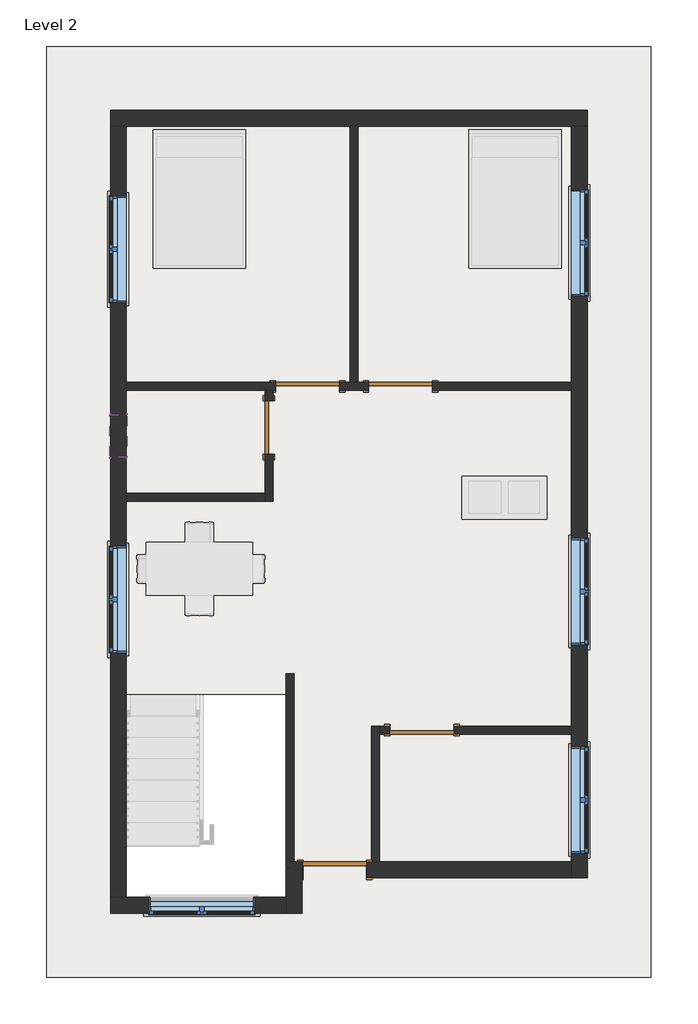
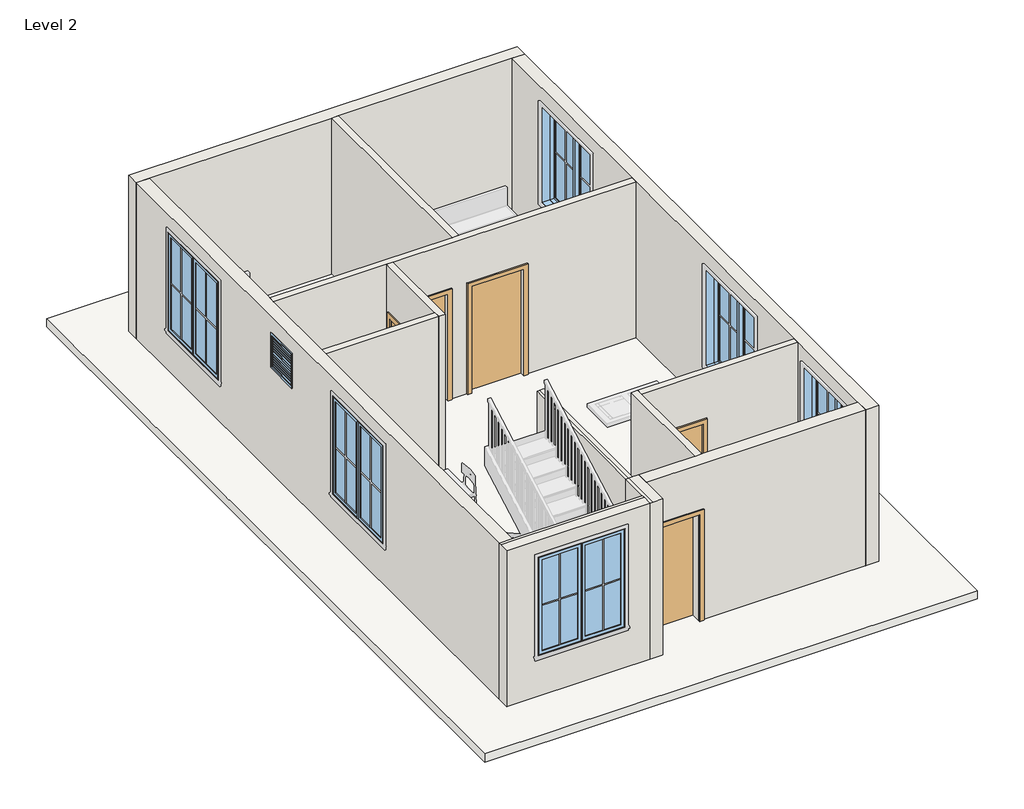
# One storey, part 1 of 3: 13 walls, 7 windows, 5 doors, 1 roof.
"""IFC4 building model written with IfcOpenShell, lengths in millimetres."""

from ifc_helpers import new_model, si_unit, frame, origin, place, context, project, spatial, polyline, outline, extrude, faceted_brep, transform, mapped, element, save
from components import door_214872d5, single_flush_door_3_e5f9f3c4, single_flush_door_3_305aa2a5, single_flush_door_3_0ca8825f, window_casement_double_win_5_f93960c7, window_f2d8fef0

model = new_model("IFC4")

# Units and contexts
model_context = context("Model", 3, world=origin())
ifc_project = project(units=[si_unit("LENGTHUNIT", "METRE", prefix="MILLI")], contexts=[model_context])

# Site, building, storey
site = spatial("IfcSite", under=ifc_project)
building = spatial("IfcBuilding", under=site)
storey = spatial("IfcBuildingStorey", under=building, Name="Level 2", Elevation=3048.0)

# Doors
placement = place(None, origin())
door_shape = door_214872d5(model_context)
element("IfcDoor", 1, ObjectType="Single-Flush : DOOR 2'6\"", at=placement, inside=storey, context=model_context, shape_type="MappedRepresentation", body=[
    mapped(door_shape, transform((-2193.930864, 251.0919982, 3048.0), x_axis=(0.0, 1.0, 0.0), y_axis=(-1.0, 0.0, 0.0), z_axis=(0.0, 0.0, 1.0))),
])
single_flush_door_3_shape = single_flush_door_3_e5f9f3c4(model_context)
element("IfcDoor", 2, ObjectType="Single-Flush : DOOR 3'", at=placement, inside=storey, context=model_context, shape_type="MappedRepresentation", body=[
    mapped(single_flush_door_3_shape, transform((-1641.3962678, 841.6419982, 3048.0), x_axis=(1.0, 0.0, 0.0), y_axis=(0.0, 1.0, 0.0), z_axis=(0.0, 0.0, 1.0))),
])
element("IfcDoor", 3, ObjectType="Single-Flush : DOOR 3'", at=placement, inside=storey, context=model_context, shape_type="MappedRepresentation", body=[
    mapped(single_flush_door_3_shape, transform((-3.180864, -4073.2580018, 3048.0), x_axis=(-1.0, 0.0, 0.0), y_axis=(0.0, -1.0, 0.0), z_axis=(0.0, 0.0, 1.0))),
])
single_flush_door_3_2_shape = single_flush_door_3_305aa2a5(model_context)
element("IfcDoor", 4, ObjectType="Single-Flush : DOOR 3'", at=placement, inside=storey, context=model_context, shape_type="MappedRepresentation", body=[
    mapped(single_flush_door_3_2_shape, transform((-307.980864, 841.6419982, 3048.0), x_axis=(-1.0, 0.0, 0.0), y_axis=(0.0, -1.0, 0.0), z_axis=(0.0, 0.0, 1.0))),
])
single_flush_door_3_3_shape = single_flush_door_3_0ca8825f(model_context)
element("IfcDoor", 5, ObjectType="Single-Flush : DOOR 3'", at=placement, inside=storey, context=model_context, shape_type="MappedRepresentation", body=[
    mapped(single_flush_door_3_3_shape, transform((-1250.955864, -6073.5080018, 3048.0), x_axis=(1.0, 0.0, 0.0), y_axis=(0.0, 1.0, 0.0), z_axis=(0.0, 0.0, 1.0))),
])

# Roof
element("IfcRoof", 6, ObjectType="ROOF 6\"", at=placement, inside=storey, context=model_context, shape_type="SweptSolid", body=[
    extrude(outline(polyline([(3273.419136, 5699.3919982), (3273.419136, -7610.2080018), (-5375.280864, -7610.2080018), (-5375.280864, 5699.3919982), (3273.419136, 5699.3919982)]), holes=[polyline([(-1895.480864, -3571.6080018), (-4232.280864, -3571.6080018), (-4232.280864, -6518.0080018), (-1895.480864, -6518.0080018), (-1895.480864, -3571.6080018)])]), frame((0.0, 0.0, 3048.0), z_axis=(0.0, 0.0, 1.0), x_axis=(1.0, 0.0, 0.0)), (0.0, 0.0, 1.0), 152.4),
])

# Walls
element("IfcWall", 7, ObjectType="WALL 4.5\"", at=placement, inside=storey, context=model_context, shape_type="SweptSolid", body=[
    extrude(outline(polyline([(-1031.880864, 898.7919982), (-1031.880864, 4556.3919982), (-917.580864, 4556.3919982), (-917.580864, 898.7919982), (-1031.880864, 898.7919982)])), frame((0.0, 0.0, 3048.0), z_axis=(0.0, 0.0, 1.0), x_axis=(1.0, 0.0, 0.0)), (0.0, 0.0, 1.0), 3048.0),
])
element("IfcWall", 8, ObjectType="WALL 4.5\"", at=placement, inside=storey, context=model_context, shape_type="Brep", body=[
    faceted_brep([(-765.180864, 898.7919982, 5181.6), (-765.180864, 898.7919982, 3048.0), (-917.580864, 898.7919982, 3048.0), (-1031.880864, 898.7919982, 3048.0), (-1184.1962678, 898.7919982, 3048.0), (-1184.1962678, 898.7919982, 5181.6), (-2098.5962678, 898.7919982, 5181.6), (-2098.5962678, 898.7919982, 3048.0), (-4232.280864, 898.7919982, 3048.0), (-4232.280864, 898.7919982, 6096.0), (-1031.880864, 898.7919982, 6096.0), (-917.580864, 898.7919982, 6096.0), (2130.419136, 898.7919982, 6096.0), (2130.419136, 898.7919982, 3048.0), (149.219136, 898.7919982, 3048.0), (149.219136, 898.7919982, 5181.6), (-1184.1962678, 784.4919982, 3048.0), (-765.180864, 784.4919982, 3048.0), (-765.180864, 784.4919982, 5181.6), (149.219136, 784.4919982, 5181.6), (149.219136, 784.4919982, 3048.0), (2130.419136, 784.4919982, 3048.0), (2130.419136, 784.4919982, 6096.0), (-2136.780864, 784.4919982, 6096.0), (-2251.080864, 784.4919982, 6096.0), (-4232.280864, 784.4919982, 6096.0), (-4232.280864, 784.4919982, 3048.0), (-2251.080864, 784.4919982, 3048.0), (-2136.780864, 784.4919982, 3048.0), (-2098.5962678, 784.4919982, 3048.0), (-2098.5962678, 784.4919982, 5181.6), (-1184.1962678, 784.4919982, 5181.6)], [[[0, 1, 2, 3, 4, 5, 6, 7, 8, 9, 10, 11, 12, 13, 14, 15]], [[16, 17, 18, 19, 20, 21, 22, 23, 24, 25, 26, 27, 28, 29, 30, 31]], [[29, 28, 27, 26, 8, 7]], [[14, 13, 21, 20]], [[4, 3, 2, 1, 17, 16]], [[13, 12, 22, 21]], [[9, 8, 26, 25]], [[5, 4, 16, 31]], [[6, 5, 31, 30]], [[7, 6, 30, 29]], [[18, 17, 1, 0]], [[19, 18, 0, 15]], [[20, 19, 15, 14]], [[12, 11, 10, 9, 25, 24, 23, 22]]]),
])
element("IfcWall", 9, ObjectType="WALL 4.5\"", at=placement, inside=storey, context=model_context, shape_type="Brep", body=[
    faceted_brep([(-2251.080864, 784.4919982, 3048.0), (-2251.080864, 632.0919982, 3048.0), (-2251.080864, 632.0919982, 5181.6), (-2251.080864, -129.9080018, 5181.6), (-2251.080864, -129.9080018, 3048.0), (-2251.080864, -688.7080018, 3048.0), (-2251.080864, -803.0080018, 3048.0), (-2251.080864, -803.0080018, 6096.0), (-2251.080864, -688.7080018, 6096.0), (-2251.080864, 784.4919982, 6096.0), (-2136.780864, 632.0919982, 5181.6), (-2136.780864, 632.0919982, 3048.0), (-2136.780864, 784.4919982, 3048.0), (-2136.780864, 784.4919982, 6096.0), (-2136.780864, -803.0080018, 6096.0), (-2136.780864, -803.0080018, 3048.0), (-2136.780864, -129.9080018, 3048.0), (-2136.780864, -129.9080018, 5181.6)], [[[0, 1, 2, 3, 4, 5, 6, 7, 8, 9]], [[10, 11, 12, 13, 14, 15, 16, 17]], [[16, 15, 6, 5, 4]], [[12, 11, 1, 0]], [[0, 9, 13, 12]], [[7, 6, 15, 14]], [[2, 1, 11, 10]], [[3, 2, 10, 17]], [[4, 3, 17, 16]], [[9, 8, 7, 14, 13]]]),
])
element("IfcWall", 10, ObjectType="WALL 4.5\"", at=placement, inside=storey, context=model_context, shape_type="SweptSolid", body=[
    extrude(outline(polyline([(-4232.280864, -688.7080018), (-2251.080864, -688.7080018), (-2251.080864, -803.0080018), (-4232.280864, -803.0080018), (-4232.280864, -688.7080018)])), frame((0.0, 0.0, 3048.0), z_axis=(0.0, 0.0, 1.0), x_axis=(1.0, 0.0, 0.0)), (0.0, 0.0, 1.0), 3048.0),
])
element("IfcWall", 11, ObjectType="WALL 4.5\"", at=placement, inside=storey, context=model_context, shape_type="Brep", body=[
    faceted_brep([(-1831.980864, -5959.2080018, 3048.0), (-1831.980864, -3266.8080018, 3048.0), (-1831.980864, -3266.8080018, 6096.0), (-1831.980864, -5959.2080018, 6096.0), (-1946.280864, -5959.2080018, 3048.0), (-1946.280864, -5959.2080018, 6096.0), (-1946.280864, -3266.8080018, 6096.0), (-1946.280864, -3266.8080018, 3048.0), (-1895.480864, -3266.8080018, 6096.0), (-1895.480864, -5959.2080018, 6096.0), (-1895.480864, -3571.6080018, 6096.0)], [[[0, 1, 2, 3]], [[4, 5, 6, 7]], [[1, 0, 4, 7]], [[2, 1, 7, 6, 8]], [[0, 3, 9, 5, 4]], [[3, 2, 8, 10, 9]], [[8, 6, 5, 9, 10]]]),
])
element("IfcWall", 12, ObjectType="WALL 4.5\"", at=placement, inside=storey, context=model_context, shape_type="Brep", body=[
    faceted_brep([(-612.780864, -5959.2080018, 3048.0), (-612.780864, -4130.4080018, 3048.0), (-612.780864, -4016.1080018, 3048.0), (-612.780864, -4016.1080018, 6096.0), (-612.780864, -4130.4080018, 6096.0), (-612.780864, -5959.2080018, 6096.0), (-727.080864, -5959.2080018, 3048.0), (-727.080864, -5959.2080018, 6096.0), (-727.080864, -4016.1080018, 6096.0), (-727.080864, -4016.1080018, 3048.0)], [[[0, 1, 2, 3, 4, 5]], [[6, 7, 8, 9]], [[2, 1, 0, 6, 9]], [[0, 5, 7, 6]], [[3, 2, 9, 8]], [[5, 4, 3, 8, 7]]]),
])
element("IfcWall", 13, ObjectType="WALL 4.5\"", at=placement, inside=storey, context=model_context, shape_type="SweptSolid", body=[
    extrude(outline(polyline([(3048.0, -612.780864), (3048.0, -460.380864), (5181.6, -460.380864), (5181.6, 454.019136), (3048.0, 454.019136), (3048.0, 2130.419136), (6096.0, 2130.419136), (6096.0, -612.780864), (3048.0, -612.780864)])), frame((0.0, -4130.4080018, 0.0), z_axis=(0.0, 1.0, 0.0), x_axis=(0.0, 0.0, 1.0)), (0.0, 0.0, 1.0), 114.3),
])
element("IfcWall", 14, ObjectType="WALL 9\"", at=placement, inside=storey, context=model_context, shape_type="Brep", body=[
    faceted_brep([(-4460.880864, 4556.3919982, 3048.0), (-4232.280864, 4556.3919982, 3048.0), (-1031.880864, 4556.3919982, 3048.0), (-917.580864, 4556.3919982, 3048.0), (2130.419136, 4556.3919982, 3048.0), (2359.019136, 4556.3919982, 3048.0), (2359.019136, 4556.3919982, 6096.0), (2130.419136, 4556.3919982, 6096.0), (-917.580864, 4556.3919982, 6096.0), (-1031.880864, 4556.3919982, 6096.0), (-4232.280864, 4556.3919982, 6096.0), (-4460.880864, 4556.3919982, 6096.0), (-4460.880864, 4784.9919982, 3048.0), (-4460.880864, 4784.9919982, 6096.0), (2359.019136, 4784.9919982, 6096.0), (2359.019136, 4784.9919982, 3048.0)], [[[0, 1, 2, 3, 4, 5, 6, 7, 8, 9, 10, 11]], [[12, 13, 14, 15]], [[5, 4, 3, 2, 1, 0, 12, 15]], [[6, 5, 15, 14]], [[0, 11, 13, 12]], [[11, 10, 9, 8, 7, 6, 14, 13]]]),
])
element("IfcWall", 15, ObjectType="WALL 9\"", at=placement, inside=storey, context=model_context, shape_type="Brep", body=[
    faceted_brep([(2130.419136, 4556.3919982, 3048.0), (2130.419136, 898.7919982, 3048.0), (2130.419136, 784.4919982, 3048.0), (2130.419136, -4016.1080018, 3048.0), (2130.419136, -4130.4080018, 3048.0), (2130.419136, -5959.2080018, 3048.0), (2130.419136, -6187.8080018, 3048.0), (2130.419136, -6187.8080018, 6096.0), (2130.419136, -5959.2080018, 6096.0), (2130.419136, -4130.4080018, 6096.0), (2130.419136, -4016.1080018, 6096.0), (2130.419136, 784.4919982, 6096.0), (2130.419136, 898.7919982, 6096.0), (2130.419136, 4556.3919982, 6096.0), (2130.419136, -5835.3830018, 5791.2), (2130.419136, -5835.3830018, 3962.4), (2130.419136, -4311.3830018, 3962.4), (2130.419136, -4311.3830018, 5791.2), (2130.419136, -2854.0580018, 5791.2), (2130.419136, -2854.0580018, 3962.4), (2130.419136, -1330.0580018, 3962.4), (2130.419136, -1330.0580018, 5791.2), (2130.419136, 2130.6919982, 5791.2), (2130.419136, 2130.6919982, 3962.4), (2130.419136, 3654.6919982, 3962.4), (2130.419136, 3654.6919982, 5791.2), (2359.019136, 4556.3919982, 3048.0), (2359.019136, 4556.3919982, 6096.0), (2359.019136, -6187.8080018, 6096.0), (2359.019136, -6187.8080018, 3048.0), (2359.019136, -5835.3830018, 5791.2), (2359.019136, -4311.3830018, 5791.2), (2359.019136, -4311.3830018, 3962.4), (2359.019136, -5835.3830018, 3962.4), (2359.019136, -2854.0580018, 5791.2), (2359.019136, -1330.0580018, 5791.2), (2359.019136, -1330.0580018, 3962.4), (2359.019136, -2854.0580018, 3962.4), (2359.019136, 2130.6919982, 5791.2), (2359.019136, 3654.6919982, 5791.2), (2359.019136, 3654.6919982, 3962.4), (2359.019136, 2130.6919982, 3962.4)], [[[0, 1, 2, 3, 4, 5, 6, 7, 8, 9, 10, 11, 12, 13], [14, 15, 16, 17], [18, 19, 20, 21], [22, 23, 24, 25]], [[26, 27, 28, 29], [30, 31, 32, 33], [34, 35, 36, 37], [38, 39, 40, 41]], [[6, 5, 4, 3, 2, 1, 0, 26, 29]], [[0, 13, 27, 26]], [[7, 6, 29, 28]], [[15, 14, 30, 33]], [[16, 15, 33, 32]], [[17, 16, 32, 31]], [[14, 17, 31, 30]], [[19, 18, 34, 37]], [[20, 19, 37, 36]], [[21, 20, 36, 35]], [[18, 21, 35, 34]], [[23, 22, 38, 41]], [[24, 23, 41, 40]], [[25, 24, 40, 39]], [[22, 25, 39, 38]], [[13, 12, 11, 10, 9, 8, 7, 28, 27]]]),
])
element("IfcWall", 16, ObjectType="WALL 9\"", at=placement, inside=storey, context=model_context, shape_type="Brep", body=[
    faceted_brep([(2130.419136, -5959.2080018, 3048.0), (-612.780864, -5959.2080018, 3048.0), (-727.080864, -5959.2080018, 3048.0), (-793.755864, -5959.2080018, 3048.0), (-793.755864, -5959.2080018, 5181.6), (-1708.155864, -5959.2080018, 5181.6), (-1708.155864, -5959.2080018, 3048.0), (-1717.680864, -5959.2080018, 3048.0), (-1717.680864, -5959.2080018, 6096.0), (-727.080864, -5959.2080018, 6096.0), (-612.780864, -5959.2080018, 6096.0), (2130.419136, -5959.2080018, 6096.0), (-793.755864, -6187.8080018, 5181.6), (-793.755864, -6187.8080018, 3048.0), (2130.419136, -6187.8080018, 3048.0), (2130.419136, -6187.8080018, 6096.0), (-1717.680864, -6187.8080018, 6096.0), (-1717.680864, -6187.8080018, 3048.0), (-1708.155864, -6187.8080018, 3048.0), (-1708.155864, -6187.8080018, 5181.6)], [[[0, 1, 2, 3, 4, 5, 6, 7, 8, 9, 10, 11]], [[12, 13, 14, 15, 16, 17, 18, 19]], [[18, 17, 7, 6]], [[14, 13, 3, 2, 1, 0]], [[0, 11, 15, 14]], [[8, 7, 17, 16]], [[4, 3, 13, 12]], [[5, 4, 12, 19]], [[6, 5, 19, 18]], [[11, 10, 9, 8, 16, 15]]]),
])
element("IfcWall", 17, ObjectType="WALL 9\"", at=placement, inside=storey, context=model_context, shape_type="Brep", body=[
    faceted_brep([(-1946.280864, -5959.2080018, 3048.0), (-1946.280864, -6467.2080018, 3048.0), (-1946.280864, -6695.8080018, 3048.0), (-1946.280864, -6695.8080018, 6096.0), (-1946.280864, -6467.2080018, 6096.0), (-1946.280864, -5959.2080018, 6096.0), (-1717.680864, -5959.2080018, 3048.0), (-1717.680864, -5959.2080018, 6096.0), (-1717.680864, -6187.8080018, 6096.0), (-1717.680864, -6695.8080018, 6096.0), (-1717.680864, -6695.8080018, 3048.0), (-1717.680864, -6187.8080018, 3048.0), (-1831.980864, -5959.2080018, 3048.0), (-1895.480864, -5959.2080018, 6096.0), (-1831.980864, -5959.2080018, 6096.0), (-1895.480864, -6695.8080018, 6096.0), (-1895.480864, -6518.0080018, 6096.0)], [[[0, 1, 2, 3, 4, 5]], [[6, 7, 8, 9, 10, 11]], [[2, 1, 0, 12, 6, 11, 10]], [[0, 5, 13, 14, 7, 6, 12]], [[3, 2, 10, 9, 15]], [[5, 4, 3, 15, 16, 13]], [[15, 9, 8, 7, 14, 13, 16]]]),
])
element("IfcWall", 18, ObjectType="WALL 9\"", at=placement, inside=storey, context=model_context, shape_type="Brep", body=[
    faceted_brep([(-1946.280864, -6467.2080018, 3048.0), (-4232.280864, -6467.2080018, 3048.0), (-4460.880864, -6467.2080018, 3048.0), (-4460.880864, -6467.2080018, 6096.0), (-4232.280864, -6467.2080018, 6096.0), (-1946.280864, -6467.2080018, 6096.0), (-3914.780864, -6467.2080018, 5791.2), (-3914.780864, -6467.2080018, 3962.4), (-2390.780864, -6467.2080018, 3962.4), (-2390.780864, -6467.2080018, 5791.2), (-1946.280864, -6695.8080018, 3048.0), (-1946.280864, -6695.8080018, 6096.0), (-4460.880864, -6695.8080018, 6096.0), (-4460.880864, -6695.8080018, 3048.0), (-3914.780864, -6695.8080018, 5791.2), (-2390.780864, -6695.8080018, 5791.2), (-2390.780864, -6695.8080018, 3962.4), (-3914.780864, -6695.8080018, 3962.4), (-1946.280864, -6518.0080018, 6096.0), (-4460.880864, -6518.0080018, 6096.0), (-4232.280864, -6518.0080018, 6096.0)], [[[0, 1, 2, 3, 4, 5], [6, 7, 8, 9]], [[10, 11, 12, 13], [14, 15, 16, 17]], [[2, 1, 0, 10, 13]], [[0, 5, 18, 11, 10]], [[3, 2, 13, 12, 19]], [[7, 6, 14, 17]], [[8, 7, 17, 16]], [[9, 8, 16, 15]], [[6, 9, 15, 14]], [[5, 4, 3, 19, 20, 18]], [[19, 12, 11, 18, 20]]]),
])
element("IfcWall", 19, ObjectType="WALL 9\"", at=placement, inside=storey, context=model_context, shape_type="Brep", body=[
    faceted_brep([(-4232.280864, -6467.2080018, 3048.0), (-4232.280864, -803.0080018, 3048.0), (-4232.280864, -688.7080018, 3048.0), (-4232.280864, 784.4919982, 3048.0), (-4232.280864, 898.7919982, 3048.0), (-4232.280864, 4556.3919982, 3048.0), (-4232.280864, 4556.3919982, 6096.0), (-4232.280864, 898.7919982, 6096.0), (-4232.280864, 784.4919982, 6096.0), (-4232.280864, -688.7080018, 6096.0), (-4232.280864, -803.0080018, 6096.0), (-4232.280864, -3571.6080018, 6096.0), (-4232.280864, -6467.2080018, 6096.0), (-4232.280864, -1445.1400081, 5791.2), (-4232.280864, -1445.1400081, 3962.4), (-4232.280864, -2969.1400081, 3962.4), (-4232.280864, -2969.1400081, 5791.2), (-4232.280864, 3562.6287133, 5791.2), (-4232.280864, 3562.6287133, 3962.4), (-4232.280864, 2038.6287133, 3962.4), (-4232.280864, 2038.6287133, 5791.2), (-4232.280864, -174.3580018, 5791.2), (-4232.280864, 435.2419982, 5791.2), (-4232.280864, 435.2419982, 5181.6), (-4232.280864, -174.3580018, 5181.6), (-4460.880864, -6467.2080018, 3048.0), (-4460.880864, -6467.2080018, 6096.0), (-4460.880864, 4556.3919982, 6096.0), (-4460.880864, 4556.3919982, 3048.0), (-4460.880864, -1445.1400081, 5791.2), (-4460.880864, -2969.1400081, 5791.2), (-4460.880864, -2969.1400081, 3962.4), (-4460.880864, -1445.1400081, 3962.4), (-4460.880864, 3562.6287133, 5791.2), (-4460.880864, 2038.6287133, 5791.2), (-4460.880864, 2038.6287133, 3962.4), (-4460.880864, 3562.6287133, 3962.4), (-4460.880864, -174.3580018, 5791.2), (-4460.880864, -174.3580018, 5181.6), (-4460.880864, 435.2419982, 5181.6), (-4460.880864, 435.2419982, 5791.2)], [[[0, 1, 2, 3, 4, 5, 6, 7, 8, 9, 10, 11, 12], [13, 14, 15, 16], [17, 18, 19, 20], [21, 22, 23, 24]], [[25, 26, 27, 28], [29, 30, 31, 32], [33, 34, 35, 36], [37, 38, 39, 40]], [[5, 4, 3, 2, 1, 0, 25, 28]], [[6, 5, 28, 27]], [[0, 12, 26, 25]], [[14, 13, 29, 32]], [[15, 14, 32, 31]], [[16, 15, 31, 30]], [[13, 16, 30, 29]], [[18, 17, 33, 36]], [[19, 18, 36, 35]], [[20, 19, 35, 34]], [[17, 20, 34, 33]], [[38, 37, 21, 24]], [[39, 38, 24, 23]], [[40, 39, 23, 22]], [[37, 40, 22, 21]], [[12, 11, 10, 9, 8, 7, 6, 27, 26]]]),
])

# Windows
window_casement_double_win_5_shape = window_casement_double_win_5_f93960c7(model_context)
element("IfcWindow", 20, ObjectType="Window-Casement-Double : WIN 5'", at=placement, inside=storey, context=model_context, shape_type="MappedRepresentation", body=[
    mapped(window_casement_double_win_5_shape, transform((-3152.780864, -6581.5080018, 3048.0), x_axis=(-1.0, 0.0, 0.0), y_axis=(0.0, -1.0, 0.0), z_axis=(0.0, 0.0, 1.0))),
])
element("IfcWindow", 21, ObjectType="Window-Casement-Double : WIN 5'", at=placement, inside=storey, context=model_context, shape_type="MappedRepresentation", body=[
    mapped(window_casement_double_win_5_shape, transform((2244.719136, -5073.3830018, 3048.0), x_axis=(0.0, -1.0, 0.0), y_axis=(1.0, 0.0, 0.0), z_axis=(0.0, 0.0, 1.0))),
])
element("IfcWindow", 22, ObjectType="Window-Casement-Double : WIN 5'", at=placement, inside=storey, context=model_context, shape_type="MappedRepresentation", body=[
    mapped(window_casement_double_win_5_shape, transform((2244.719136, -2092.0580018, 3048.0), x_axis=(0.0, -1.0, 0.0), y_axis=(1.0, 0.0, 0.0), z_axis=(0.0, 0.0, 1.0))),
])
element("IfcWindow", 23, ObjectType="Window-Casement-Double : WIN 5'", at=placement, inside=storey, context=model_context, shape_type="MappedRepresentation", body=[
    mapped(window_casement_double_win_5_shape, transform((-4346.580864, -2207.1400081, 3048.0), x_axis=(0.0, 1.0, 0.0), y_axis=(-1.0, 0.0, 0.0), z_axis=(0.0, 0.0, 1.0))),
])
element("IfcWindow", 24, ObjectType="Window-Casement-Double : WIN 5'", at=placement, inside=storey, context=model_context, shape_type="MappedRepresentation", body=[
    mapped(window_casement_double_win_5_shape, transform((2244.719136, 2892.6919982, 3048.0), x_axis=(0.0, -1.0, 0.0), y_axis=(1.0, 0.0, 0.0), z_axis=(0.0, 0.0, 1.0))),
])
element("IfcWindow", 25, ObjectType="Window-Casement-Double : WIN 5'", at=placement, inside=storey, context=model_context, shape_type="MappedRepresentation", body=[
    mapped(window_casement_double_win_5_shape, transform((-4346.580864, 2800.6287133, 3048.0), x_axis=(0.0, 1.0, 0.0), y_axis=(-1.0, 0.0, 0.0), z_axis=(0.0, 0.0, 1.0))),
])
window_shape = window_f2d8fef0(model_context)
element("IfcWindow", 26, ObjectType="Window-Louvers : 24\" x 24\"", at=placement, inside=storey, context=model_context, shape_type="MappedRepresentation", body=[
    mapped(window_shape, transform((-4352.930864, 130.4419982, 4267.2), x_axis=(0.0, 1.0, 0.0), y_axis=(-1.0, 0.0, 0.0), z_axis=(0.0, 0.0, 1.0))),
])

save(model, "model.ifc")

# Revit data of these elements
# Type "Single-Flush : DOOR 2'6\""
#   Type Mark = "9"
#   Construction Type Id = "MDOOR"
#   Assembly Code = "C1020"
#   Analytic Construction = "Metal"
#   Thickness = 0' - 2"
#   Heat Transfer Coefficient (U) = 0.651978 BTU/(h·ft²·°F)
#   Height = 7' - 0"
#   Trim Projection Ext = 0' - 1"
#   Trim Projection Int = 0' - 1"
#   Trim Width = 0' - 3"
#   Width = 2' - 6"
#   Define Thermal Properties by = 1
#   Door Material = Door - Panel
#   Frame Material = Door - Frame
#   Visual Light Transmittance = 0
#   Solar Heat Gain Coefficient = 0
#   Function = (empty or 0)
#   Wall Closure = (empty or 0)
# Type "Single-Flush : DOOR 3'"
#   Type Mark = "8"
#   Construction Type Id = "MDOOR"
#   Assembly Code = "C1020"
#   Analytic Construction = "Metal"
#   Thickness = 0' - 2"
#   Heat Transfer Coefficient (U) = 0.651978 BTU/(h·ft²·°F)
#   Height = 7' - 0"
#   Trim Projection Ext = 0' - 1"
#   Trim Projection Int = 0' - 1"
#   Trim Width = 0' - 3"
#   Width = 3' - 0"
#   Define Thermal Properties by = 1
#   Door Material = Door - Panel
#   Frame Material = Door - Frame
#   Visual Light Transmittance = 0
#   Solar Heat Gain Coefficient = 0
#   Function = (empty or 0)
#   Wall Closure = (empty or 0)
# Type "ROOF 6\""
#   Assembly Code = "B1020"
#   Layers, outside or top first: 0' - 6" no material (function 1)
# Type "WALL 4.5\""
#   Assembly Code = "B2010"
#   Layers, outside or top first: 0' - 4 1/2" no material (function 1)
# Type "WALL 9\""
#   Assembly Code = "B2010"
#   Layers, outside or top first: 0' - 9" no material (function 1)
# Type "Window-Casement-Double : WIN 5'"
#   Type Mark = "18"
#   Fire Rating = "0.5h"
#   Assembly Code = "B2020100"
#   Analytic Construction = "Double glazing - domestic"
#   Frame Extension [instance default] = 0' - 0 1/4"
#   Window Inset [instance default] = 0' - 0"
#   Wall Thickness [instance default] = 0' - 6"
#   Interior Wall Closure [instance default] = 0' - 2 1/4"
#   Half Width = 2' - 6"
#   Visual Light Transmittance = 0.81
#   Thermal Resistance (R) = 1.8146 (h·ft²·°F)/BTU
#   Solar Heat Gain Coefficient = 0.76
#   Rough Width = 5' - 0 1/2"
#   Rough Height = 6' - 0 1/2"
#   Height = 6' - 0"
#   Heat Transfer Coefficient (U) = 0.5511 BTU/(h·ft²·°F)
#   Exterior Wall Closure [instance default] = 0' - 1 1/4"
#   Extension Jamb [instance default] = 0' - 2 1/4"
#   Default Sill Height = 3' - 0"
#   Width = 5' - 0"
#   Muntin Visibility = yes
#   Interior Trim Visibility [instance default] = yes
#   Exterior Trim Visibility [instance default] = yes
#   Extension Jamb Visibility [instance default] = yes
#   Interior Trim Material = Wood - Stained
#   Muntin Pattern = Muntin Pattern_2x2 : Muntin Pattern_2x2
#   Interior Trim = Trim-Window-Interior-Flat : Picture Frame
#   Interior Frame Material = Wood - Stained
#   Glass Panel Material = Glass
#   Exterior Trim Material = Clad - White
#   Exterior Trim = Trim-Window-Exterior-Flat : with Sill
#   Exterior Frame Material = Clad - White
#   Wall Closure = (empty or 0)
# Type "Window-Louvers : 24\" x 24\""
#   Type Mark = "19"
#   Construction Type Id = "GSP4R"
#   Assembly Code = "B20"
#   Analytic Construction = "1/8 in Pilkington single glazing"
#   Visual Light Transmittance = 0.9
#   Thermal Resistance (R) = 1.53941 (h·ft²·°F)/BTU
#   Solar Heat Gain Coefficient = 0.78
#   Max Height = 1' - 11.74264"
#   Height = 2' - 0"
#   Heat Transfer Coefficient (U) = 0.6496 BTU/(h·ft²·°F)
#   Blade Width [instance default] = 1' - 10 1/2"
#   Blade Vertical Thickness = 0' - 0.35355"
#   Blade Thickness = 0' - 0 1/4"
#   Blade Spacing = 0' - 1 1/2"
#   Blade Height = 0' - 1.85355"
#   Blade Depth = 0' - 3"
#   Blade Angle = 45.00°
#   Default Sill Height = 3' - 0"
#   Trim Projection_Exterior = 0' - 0 1/2"
#   Trim Projection_Interior = 0' - 0 1/2"
#   Trim Width_Exterior = 0' - 1 1/2"
#   Trim Width_Interior = 0' - 1 1/2"
#   Width = 2' - 0"
#   Max Blade Count = 12
#   Define Thermal Properties by = 1
#   Blade Count = 12
#   Frame Material = Birch
#   Louver Material = Birch
#   Trim Exterior Material = Birch
#   Trim Interior Material = Birch
#   Wall Closure = (empty or 0)
# Element 1 (IfcDoor, "Single-Flush : DOOR 2'6\"")
#   Phase Created = New Construction
#   Materials on its faces: "Door - Frame", "Door - Panel"
# Elements 2, 3, 4, 5 (IfcDoor, "Single-Flush : DOOR 3'")
#   Phase Created = New Construction
#   Materials on its faces: "Door - Frame", "Door - Panel"
# Element 6 (IfcRoof, "ROOF 6\"")
#   built-in parameter 1001705 = 10.5 (stored number, unit not read)
#   built-in parameter 1001710 = 33615
#   Phase Created = New Construction
#   Materials on its faces: "Copper", "Wood - Stained"
# Elements 7, 8, 9, 10, 12, 13 (IfcWall, "WALL 4.5\"")
#   Top Offset = 0' - 0"
#   Base Offset = 0' - 0"
#   Unconnected Height = 10' - 0"
#   wall height = 10' - 0"
#   Phase Created = New Construction
#   Base Constraint = Level 2
#   Materials on its faces: "Default Wall"
# Element 11 (IfcWall, "WALL 4.5\"")
#   Top Offset = 0' - 0"
#   Base Offset = 0' - 0"
#   Unconnected Height = 10' - 0"
#   wall height = 10' - 0"
#   Phase Created = New Construction
#   Base Constraint = Level 2
#   Materials on its faces: "Default Wall", "Copper"
# Elements 14, 15, 16 (IfcWall, "WALL 9\"")
#   Top Offset = 0' - 0"
#   Base Offset = 0' - 0"
#   Unconnected Height = 10' - 0"
#   wall height = 10' - 0"
#   Phase Created = New Construction
#   Base Constraint = Level 2
#   Materials on its faces: "Default Wall"
# Elements 17, 18, 19 (IfcWall, "WALL 9\"")
#   Top Offset = 0' - 0"
#   Base Offset = 0' - 0"
#   Unconnected Height = 10' - 0"
#   wall height = 10' - 0"
#   Phase Created = New Construction
#   Base Constraint = Level 2
#   Materials on its faces: "Default Wall", "Copper"
# Element 20 (IfcWindow, "Window-Casement-Double : WIN 5'")
#   Mark = "8"
#   Window Inset = 0' - 0"
#   Interior Wall Closure = 0' - 2 1/4"
#   Frame Extension = 0' - 0 1/4"
#   Exterior Wall Closure = 0' - 1 1/4"
#   Interior Trim Visibility = yes
#   Exterior Trim Visibility = yes
#   Phase Created = New Construction
#   Materials on its faces: "Wood - Stained", "Glass", "Clad - White"
# Element 21 (IfcWindow, "Window-Casement-Double : WIN 5'")
#   Mark = "9"
#   Window Inset = 0' - 0"
#   Interior Wall Closure = 0' - 2 1/4"
#   Frame Extension = 0' - 0 1/4"
#   Exterior Wall Closure = 0' - 1 1/4"
#   Interior Trim Visibility = yes
#   Exterior Trim Visibility = yes
#   Phase Created = New Construction
#   Materials on its faces: "Wood - Stained", "Glass", "Clad - White"
# Element 22 (IfcWindow, "Window-Casement-Double : WIN 5'")
#   Mark = "10"
#   Window Inset = 0' - 0"
#   Interior Wall Closure = 0' - 2 1/4"
#   Frame Extension = 0' - 0 1/4"
#   Exterior Wall Closure = 0' - 1 1/4"
#   Interior Trim Visibility = yes
#   Exterior Trim Visibility = yes
#   Phase Created = New Construction
#   Materials on its faces: "Wood - Stained", "Glass", "Clad - White"
# Element 23 (IfcWindow, "Window-Casement-Double : WIN 5'")
#   Mark = "11"
#   Window Inset = 0' - 0"
#   Interior Wall Closure = 0' - 2 1/4"
#   Frame Extension = 0' - 0 1/4"
#   Exterior Wall Closure = 0' - 1 1/4"
#   Interior Trim Visibility = yes
#   Exterior Trim Visibility = yes
#   Phase Created = New Construction
#   Materials on its faces: "Wood - Stained", "Glass", "Clad - White"
# Element 24 (IfcWindow, "Window-Casement-Double : WIN 5'")
#   Mark = "12"
#   Window Inset = 0' - 0"
#   Interior Wall Closure = 0' - 2 1/4"
#   Frame Extension = 0' - 0 1/4"
#   Exterior Wall Closure = 0' - 1 1/4"
#   Interior Trim Visibility = yes
#   Exterior Trim Visibility = yes
#   Phase Created = New Construction
#   Materials on its faces: "Wood - Stained", "Glass", "Clad - White"
# Element 25 (IfcWindow, "Window-Casement-Double : WIN 5'")
#   Mark = "13"
#   Window Inset = 0' - 0"
#   Interior Wall Closure = 0' - 2 1/4"
#   Frame Extension = 0' - 0 1/4"
#   Exterior Wall Closure = 0' - 1 1/4"
#   Interior Trim Visibility = yes
#   Exterior Trim Visibility = yes
#   Phase Created = New Construction
#   Materials on its faces: "Wood - Stained", "Glass", "Clad - White"
# Element 26 (IfcWindow, "Window-Louvers : 24\" x 24\"")
#   Mark = "14"
#   Blade Width = 1' - 10 1/2"
#   Phase Created = New Construction
#   Materials on its faces: "Birch"
# Materials
#   "Door - Panel": class "Wood", colour RGB 210 159 95, transparency 0, Cost = 0
#   "Door - Frame": colour RGB 118 70 51, transparency 0, Cost = 0
#   "Wood - Stained": class "Wood", colour RGB 224 178 126, transparency 0, Cost = 0
#   "Glass": class "Glass", colour RGB 0 128 192, transparency 0.75, Description = "Soda Lime Glass", Cost = 0
#   "Clad - White": class "Wood", colour RGB 242 242 238, transparency 0, Cost = 0
#   "Birch": class "Wood", colour RGB 224 178 126, transparency 0, Description = "Betula Alleghaniensis", Cost = 0
#   "Copper": class "Metal", colour RGB 0 0 0, transparency 0, Description = "Copper, matte finish", Cost = 0
#   "Default Wall": colour RGB 128 128 128, transparency 0, Cost = 0
